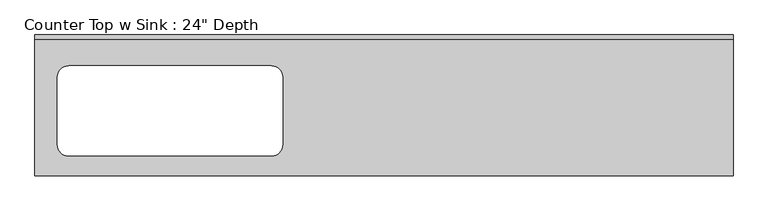
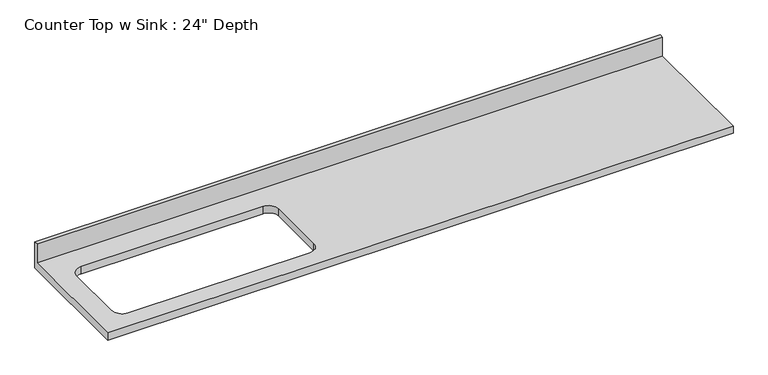
"""IFC4 building model written with IfcOpenShell, lengths in millimetres: furniture geometry."""

from ifc_helpers import new_model, si_unit, frame, origin, place, context, project, spatial, polyline, circle_curve, source, transform, mapped, element, save
from ifc_brep_helpers import plane_surface, revolved_surface, advanced_brep


def furniture_23ec23c8(model_context):
    return source(origin(), model_context, "Body", "AdvancedBrep", [
        advanced_brep(
        [(-1200.4622951, -635.0, 914.4), (1949.1377049, -635.0, 914.4), (1949.1377049, -19.05, 914.4), (-1200.4622951, -19.05, 914.4), (-1048.0622951, -139.7, 914.4), (-133.6622951, -139.7, 914.4), (-82.8622951, -190.5, 914.4), (-82.8622951, -495.3, 914.4), (-133.6622951, -546.1, 914.4), (-1048.0622951, -546.1, 914.4), (-1098.8622951, -495.3, 914.4), (-1098.8622951, -190.5, 914.4), (1949.1377049, 0.0, 876.3), (1949.1377049, -635.0, 876.3), (-1200.4622951, -635.0, 876.3), (-1200.4622951, 0.0, 876.3), (-133.6622951, -139.7, 876.3), (-1048.0622951, -139.7, 876.3), (-1098.8622951, -190.5, 876.3), (-1098.8622951, -495.3, 876.3), (-1048.0622951, -546.1, 876.3), (-133.6622951, -546.1, 876.3), (-82.8622951, -495.3, 876.3), (-82.8622951, -190.5, 876.3), (-1200.4622951, 0.0, 1016.0), (1949.1377049, 0.0, 1016.0), (-1200.4622951, -19.05, 1016.0), (1949.1377049, -19.05, 1016.0)],
        [
            (0, 1),
            (1, 2),
            (2, 3),
            (3, 0),
            (4, 5),
            (5, 6, circle_curve(frame((-133.6622951, -190.5, 914.4), z_axis=(0.0, 0.0, -1.0), x_axis=(1.0, 0.0, 0.0)), 50.8)),
            (6, 7),
            (7, 8, circle_curve(frame((-133.6622951, -495.3, 914.4), z_axis=(0.0, 0.0, -1.0), x_axis=(1.0, 0.0, 0.0)), 50.8)),
            (8, 9),
            (9, 10, circle_curve(frame((-1048.0622951, -495.3, 914.4), z_axis=(0.0, 0.0, -1.0), x_axis=(1.0, 0.0, 0.0)), 50.8)),
            (10, 11),
            (11, 4, circle_curve(frame((-1048.0622951, -190.5, 914.4), z_axis=(0.0, 0.0, -1.0), x_axis=(1.0, 0.0, 0.0)), 50.8)),
            (12, 13),
            (13, 14),
            (14, 15),
            (15, 12),
            (16, 17),
            (17, 18, circle_curve(frame((-1048.0622951, -190.5, 876.3), z_axis=(0.0, 0.0, 1.0), x_axis=(1.0, 0.0, 0.0)), 50.8)),
            (18, 19),
            (19, 20, circle_curve(frame((-1048.0622951, -495.3, 876.3), z_axis=(0.0, 0.0, 1.0), x_axis=(1.0, 0.0, 0.0)), 50.8)),
            (20, 21),
            (21, 22, circle_curve(frame((-133.6622951, -495.3, 876.3), z_axis=(0.0, 0.0, 1.0), x_axis=(1.0, 0.0, 0.0)), 50.8)),
            (22, 23),
            (23, 16, circle_curve(frame((-133.6622951, -190.5, 876.3), z_axis=(0.0, 0.0, 1.0), x_axis=(1.0, 0.0, 0.0)), 50.8)),
            (15, 24),
            (24, 25),
            (25, 12),
            (14, 0),
            (3, 26),
            (26, 24),
            (13, 1),
            (25, 27),
            (27, 2),
            (26, 27),
            (4, 17),
            (16, 5),
            (11, 18),
            (10, 19),
            (9, 20),
            (8, 21),
            (7, 22),
            (6, 23),
        ],
        [
            plane_surface(frame((-1200.4622951, 0.0, 914.4), z_axis=(0.0, 0.0, 1.0), x_axis=(-1.0, 0.0, 0.0))),
            plane_surface(frame((-1200.4622951, 0.0, 876.3), z_axis=(0.0, 0.0, -1.0), x_axis=(1.0, 0.0, 0.0))),
            plane_surface(frame((1949.1377049, 0.0, 914.4), z_axis=(0.0, 1.0, 0.0), x_axis=(0.0, 0.0, -1.0))),
            plane_surface(frame((-1200.4622951, 0.0, 914.4), z_axis=(-1.0, 0.0, 0.0), x_axis=(0.0, 0.0, -1.0))),
            plane_surface(frame((-1200.4622951, -635.0, 914.4), z_axis=(0.0, -1.0, 0.0), x_axis=(0.0, 0.0, -1.0))),
            plane_surface(frame((1949.1377049, -635.0, 914.4), z_axis=(1.0, 0.0, 0.0), x_axis=(0.0, 0.0, -1.0))),
            plane_surface(frame((-1200.4622951, 0.0, 1016.0), z_axis=(0.0, 0.0, 1.0), x_axis=(0.0, -1.0, 0.0))),
            plane_surface(frame((-1200.4622951, -19.05, 1016.0), z_axis=(0.0, -1.0, 0.0), x_axis=(0.0, 0.0, -1.0))),
            plane_surface(frame((-133.6622951, -139.7, 914.4), z_axis=(0.0, -1.0, 0.0), x_axis=(0.0, 0.0, -1.0))),
            revolved_surface(polyline([(-997.2622951000001, -190.5, 914.4), (-997.2622951000001, -190.5, 876.3)]), (-1048.0622951, -190.5, 876.3), (0.0, 0.0, 1.0)),
            plane_surface(frame((-1098.8622951, -190.5, 914.4), z_axis=(1.0, 0.0, 0.0), x_axis=(0.0, 0.0, -1.0))),
            revolved_surface(polyline([(-997.2622951000001, -495.3, 914.4), (-997.2622951000001, -495.3, 876.3)]), (-1048.0622951, -495.3, 876.3), (0.0, 0.0, 1.0)),
            plane_surface(frame((-1048.0622951, -546.1, 914.4), z_axis=(0.0, 1.0, 0.0), x_axis=(0.0, 0.0, -1.0))),
            revolved_surface(polyline([(-82.8622951, -495.3, 914.4), (-82.8622951, -495.3, 876.3)]), (-133.6622951, -495.3, 876.3), (0.0, 0.0, 1.0)),
            plane_surface(frame((-82.8622951, -495.3, 914.4), z_axis=(-1.0, 0.0, 0.0), x_axis=(0.0, 0.0, -1.0))),
            revolved_surface(polyline([(-82.8622951, -190.5, 914.4), (-82.8622951, -190.5, 876.3)]), (-133.6622951, -190.5, 876.3), (0.0, 0.0, 1.0)),
        ],
        [
            (0, [[1, 2, 3, 4], [5, 6, 7, 8, 9, 10, 11, 12]]),
            (1, [[13, 14, 15, 16], [17, 18, 19, 20, 21, 22, 23, 24]]),
            (2, [[-16, 25, 26, 27]]),
            (3, [[-15, 28, -4, 29, 30, -25]]),
            (4, [[-1, -28, -14, 31]]),
            (5, [[-13, -27, 32, 33, -2, -31]]),
            (6, [[-30, 34, -32, -26]]),
            (7, [[-34, -29, -3, -33]]),
            (8, [[35, -17, 36, -5]]),
            (9, [[-35, -12, 37, -18]]),
            (10, [[-37, -11, 38, -19]]),
            (11, [[-38, -10, 39, -20]]),
            (12, [[-39, -9, 40, -21]]),
            (13, [[-40, -8, 41, -22]]),
            (14, [[-41, -7, 42, -23]]),
            (15, [[-36, -24, -42, -6]]),
        ],
    ),
    ])


if __name__ == "__main__":
    model = new_model("IFC4")
    model_context = context("Model", 3, world=origin())
    ifc_project = project(units=[si_unit("LENGTHUNIT", "METRE", prefix="MILLI")], contexts=[model_context])
    site = spatial("IfcSite", under=ifc_project)
    building = spatial("IfcBuilding", under=site)
    placement = place(None, origin())
    furniture_shape = furniture_23ec23c8(model_context)
    element("IfcFurniture", 1, ObjectType="Counter Top w Sink : 24\" Depth", at=placement, inside=building, context=model_context, shape_type="MappedRepresentation", body=[
        mapped(furniture_shape, transform((0.0, 0.0, 0.0), x_axis=(1.0, 0.0, 0.0), y_axis=(0.0, 1.0, 0.0), z_axis=(0.0, 0.0, 1.0))),
    ])
    save(model, "model.ifc")

# Revit data of these elements
# Type "Counter Top w Sink : 24\" Depth"
#   Assembly Code = "C1030400"
#   Counter Thickness = 0' - 1 1/2"
#   Depth = 2' - 1"
#   Height = 3' - 0"
#   Length [instance default] = 8' - 0"
#   Sink Location [instance default] = 2' - 0"
#   Sink Location To Wall [instance default] = 0' - 6"
#   Sink Opening Depth [instance default] = 1' - 3"
#   Sink Opening Width [instance default] = 3' - 3"
#   Counter Top Material = none
#   Default Elevation = 0
# Element 1 (IfcFurniture, "Counter Top w Sink : 24\" Depth")
#   Length = 10' - 4"
#   Materials on its faces: "Counter Top"
# Materials
#   "Counter Top": class "Wood", colour RGB 226 177 128, transparency 0
